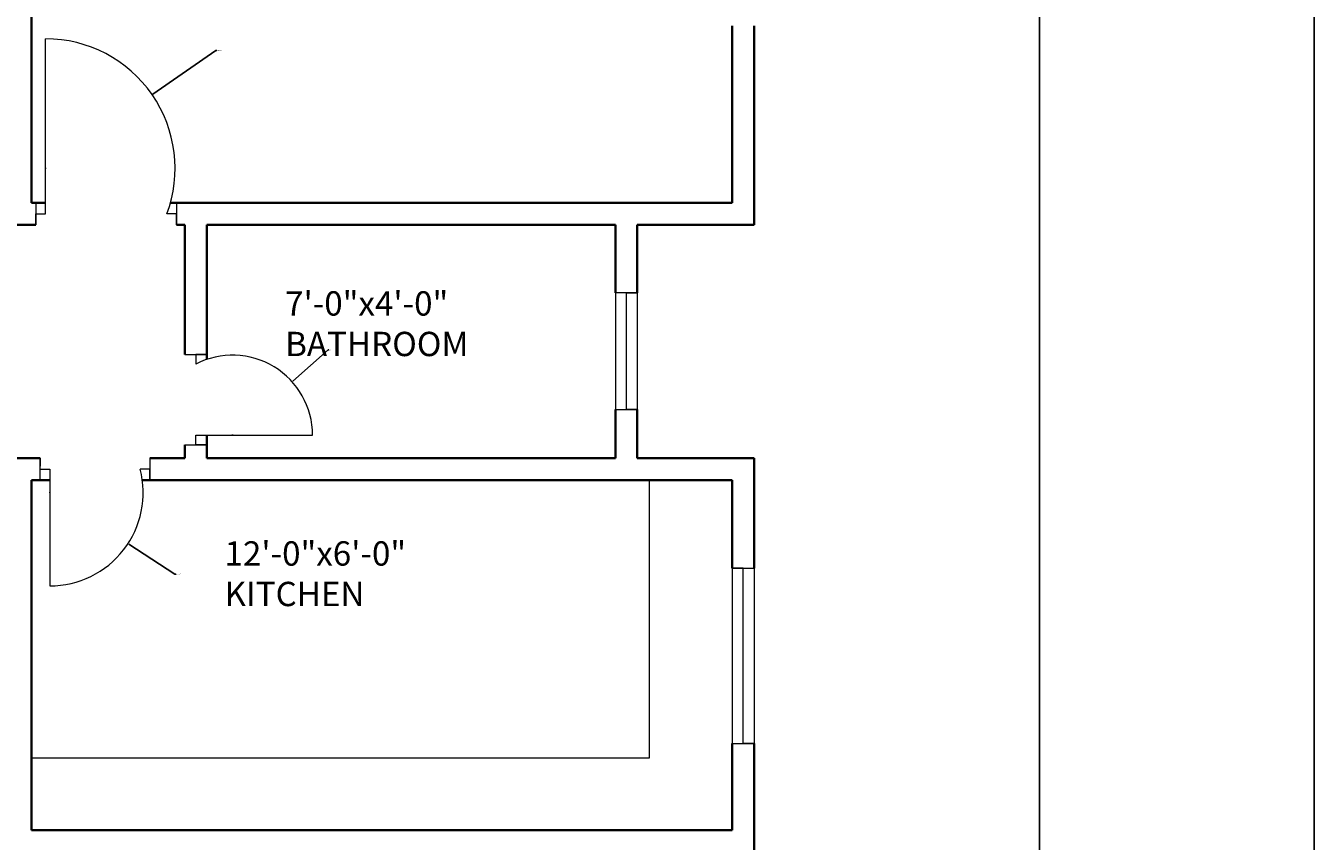
# Model space of a CAD drawing. Units: inches. Extents: x 2163 to 2982, y 1024 to 2288.
# Tile 21 of 22: x 2718 to 2982, y 1885 to 2053. Entities that reach past the tile are written whole.
import ezdxf

# ---------------------------------------------------------------- set-up
doc = ezdxf.new("R2010")
doc.units = ezdxf.units.IN
for name, color, linetype, lineweight in [('A-ANNO-DIMS', 2, 'Continuous', 18), ('A-ANNO-TTLB', 7, 'Continuous', 25), ('A-AREA-IDEN', 7, 'Continuous', 18), ('A-DOOR', 11, 'Continuous', 18), ('A-FLOR-FIXT', 9, 'Continuous', 18), ('A-GLAZ', 161, 'Continuous', 18), ('A-WALL', 7, 'Continuous', 35)]:
    doc.layers.add(name, color=color, linetype=linetype, lineweight=lineweight)
doc.styles.get("Standard").update_dxf_attribs({"font": 'arial.ttf'})
doc.dimstyles.get("Standard").update_dxf_attribs({"dimtxt": 0.18, "dimasz": 0.18, "dimexe": 0.18, "dimexo": 0.0625, "dimgap": 0.09, "dimtad": 0, "dimtih": 1, "dimtoh": 1, "dimdec": 4, "dimzin": 0, "dimdsep": 46, "dimtxsty": 'Standard', "dimcen": 0.09, "dimadec": 0, "dimazin": 0, "dimtfac": 1, "dimtdec": 4, "dimtofl": 0, "dimtmove": 0, "dimatfit": 3, "dimfxl": 1, "dimtolj": 1, "dimtzin": 0, "dimarcsym": 0})

# ---------------------------------------------------------------- blocks, each defined once
blk = doc.blocks.new('WIN-36')
for p, q in [((2.25, 36), (0, 36)), ((0, 36), (4.5, 36)), ((0, 36), (0, 0)), ((2.25, 0), (2.25, 36)), ((4.5, 36), (4.5, 0)), ((0, 0), (4.5, 0)), ((4.5, 0), (2.25, 0))]:
    blk.add_line(p, q)
blk = doc.blocks.new('*D29')
at = {"layer": 'A-ANNO-DIMS', "color": 0, "lineweight": -2, "transparency": 16777216}
for p, q in [((2285.34, 1738.83), (2285.34, 2288.1)), ((2867.34, 2229.33), (2867.34, 2288.1)), ((2285.52, 2287.92), (2576.05, 2287.92)), ((2867.16, 2287.92), (2576.63, 2287.92))]:
    blk.add_line(p, q, dxfattribs=at)
at = {"layer": 'A-ANNO-DIMS', "color": 0, "transparency": 16777216}
for points in [[(2285.52, 2287.95), (2285.52, 2287.89), (2285.34, 2287.92)], [(2867.16, 2287.95), (2867.16, 2287.89), (2867.34, 2287.92)]]:
    blk.add_solid(points, dxfattribs=at)
at = {"layer": 'Defpoints', "color": 0, "transparency": 16777216}
for p in [(2867.34, 2287.92), (2867.34, 2229.27), (2285.34, 1738.77)]:
    blk.add_point(p, dxfattribs=at)
at = {"layer": 'A-ANNO-DIMS', "color": 0, "transparency": 16777216, "insert": (2576.34, 2287.92), "char_height": 0.18, "attachment_point": 5}
blk.add_mtext('\\A1;582', dxfattribs=at)
blk = doc.blocks.new('*D31')
at = {"layer": 'A-ANNO-DIMS', "color": 0, "lineweight": -2, "transparency": 16777216}
for p, q in [((2867.4, 2229.27), (2926.17, 2229.27)), ((2925.99, 2229.09), (2925.99, 1957.95)), ((2925.99, 1686.45), (2925.99, 1957.59)), ((2862.9, 1686.27), (2926.17, 1686.27))]:
    blk.add_line(p, q, dxfattribs=at)
at = {"layer": 'A-ANNO-DIMS', "color": 0, "transparency": 16777216}
for points in [[(2925.96, 2229.09), (2926.02, 2229.09), (2925.99, 2229.27)], [(2925.96, 1686.45), (2926.02, 1686.45), (2925.99, 1686.27)]]:
    blk.add_solid(points, dxfattribs=at)
at = {"layer": 'Defpoints', "color": 0, "transparency": 16777216}
for p in [(2867.34, 2229.27), (2925.99, 2229.27), (2862.84, 1686.27)]:
    blk.add_point(p, dxfattribs=at)
at = {"layer": 'A-ANNO-DIMS', "color": 0, "transparency": 16777216, "insert": (2925.99, 1957.77), "char_height": 0.18, "attachment_point": 5}
blk.add_mtext('\\A1;543', dxfattribs=at)
blk = doc.blocks.new('*D32')
at = {"layer": 'A-ANNO-DIMS', "color": 0, "lineweight": -2, "transparency": 16777216}
for p, q in [((2867.4, 2229.27), (2926.17, 2229.27)), ((2925.99, 2229.09), (2925.99, 1686.35)), ((2925.99, 1143.25), (2925.99, 1685.99)), ((2867.4, 1143.07), (2926.17, 1143.07))]:
    blk.add_line(p, q, dxfattribs=at)
at = {"layer": 'A-ANNO-DIMS', "color": 0, "transparency": 16777216}
for points in [[(2925.96, 2229.09), (2926.02, 2229.09), (2925.99, 2229.27)], [(2925.96, 1143.25), (2926.02, 1143.25), (2925.99, 1143.07)]]:
    blk.add_solid(points, dxfattribs=at)
at = {"layer": 'Defpoints', "color": 0, "transparency": 16777216}
for p in [(2867.34, 2229.27), (2925.99, 2229.27), (2867.34, 1143.07)]:
    blk.add_point(p, dxfattribs=at)
at = {"layer": 'A-ANNO-DIMS', "color": 0, "transparency": 16777216, "insert": (2925.99, 1686.17), "char_height": 0.18, "attachment_point": 5}
blk.add_mtext('\\A1;1086.2', dxfattribs=at)
blk = doc.blocks.new('*D52')
at = {"layer": 'A-ANNO-DIMS', "color": 0, "lineweight": -2, "transparency": 16777216}
for p, q in [((2756.74, 2047.63), (2743.76, 2038.65)), ((2756.92, 2047.63), (2756.74, 2047.63)), ((2721.63, 2023.4), (2721.81, 2023.4)), ((2721.72, 2023.31), (2721.72, 2023.49))]:
    blk.add_line(p, q, dxfattribs=at)
at = {"layer": 'A-ANNO-DIMS', "color": 0, "transparency": 16777216}
blk.add_solid([(2743.74, 2038.67), (2743.78, 2038.62), (2743.61, 2038.55)], dxfattribs=at)
at = {"layer": 'Defpoints', "color": 0, "transparency": 16777216}
for p in [(2743.61, 2038.55), (2721.72, 2023.4)]:
    blk.add_point(p, dxfattribs=at)
at = {"layer": 'A-ANNO-DIMS', "color": 0, "transparency": 16777216, "insert": (2757.47, 2047.63), "char_height": 0.18, "attachment_point": 5}
blk.add_mtext('\\A1;R26.616', dxfattribs=at)
blk = doc.blocks.new('*D70')
at = {"layer": 'A-ANNO-DIMS', "color": 0, "lineweight": -2, "transparency": 16777216}
for p, q in [((2779.77, 1986.04), (2772.55, 1979.6)), ((2779.95, 1986.04), (2779.77, 1986.04)), ((2760.08, 1968.55), (2760.26, 1968.55)), ((2760.17, 1968.46), (2760.17, 1968.64))]:
    blk.add_line(p, q, dxfattribs=at)
at = {"layer": 'A-ANNO-DIMS', "color": 0, "transparency": 16777216}
blk.add_solid([(2772.53, 1979.62), (2772.57, 1979.58), (2772.42, 1979.48)], dxfattribs=at)
at = {"layer": 'Defpoints', "color": 0, "transparency": 16777216}
for p in [(2772.42, 1979.48), (2760.17, 1968.55)]:
    blk.add_point(p, dxfattribs=at)
at = {"layer": 'A-ANNO-DIMS', "color": 0, "transparency": 16777216, "insert": (2780.5, 1986.04), "char_height": 0.18, "attachment_point": 5}
blk.add_mtext('\\A1;R16.423', dxfattribs=at)
blk = doc.blocks.new('*D72')
at = {"layer": 'A-ANNO-DIMS', "color": 0, "lineweight": -2, "transparency": 16777216}
for p, q in [((2722.5, 1956.72), (2722.68, 1956.72)), ((2722.59, 1956.63), (2722.59, 1956.81)), ((2748.31, 1939.92), (2738.81, 1946.12)), ((2748.49, 1939.92), (2748.31, 1939.92))]:
    blk.add_line(p, q, dxfattribs=at)
at = {"layer": 'A-ANNO-DIMS', "color": 0, "transparency": 16777216}
blk.add_solid([(2738.83, 1946.15), (2738.8, 1946.1), (2738.66, 1946.22)], dxfattribs=at)
at = {"layer": 'Defpoints', "color": 0, "transparency": 16777216}
for p in [(2722.59, 1956.72), (2738.66, 1946.22)]:
    blk.add_point(p, dxfattribs=at)
at = {"layer": 'A-ANNO-DIMS', "color": 0, "transparency": 16777216, "insert": (2749.04, 1939.92), "char_height": 0.18, "attachment_point": 5}
blk.add_mtext('\\A1;R19.197', dxfattribs=at)

msp = doc.modelspace()

# ---------------------------------------------------------------- linework, layer by layer
at = {"layer": 'A-ANNO-TTLB'}
msp.add_lwpolyline([(2162.6841, 2274.6054), (2982.469, 2274.6054), (2982.469, 1045.9691), (2162.6841, 1045.9691)], close=True, dxfattribs=at)
at = {"layer": 'A-DOOR'}
for p, q in [((2721.7236, 2014.0188), (2721.7236, 2050.0188)), ((2719.7237, 2016.2688), (2719.7237, 2011.7688)), ((2748.6306, 2016.2688), (2748.6306, 2011.7688)), ((2719.7237, 2011.7688), (2719.7237, 2014.0188)), ((2719.7237, 2014.0188), (2721.7236, 2014.0188)), ((2748.6306, 2014.0188), (2746.6306, 2014.0188)), ((2748.6306, 2011.7688), (2748.6306, 2014.0188)), ((2750.3389, 1985.1163), (2754.8389, 1985.1163)), ((2754.8389, 1985.1163), (2752.5889, 1985.1163)), ((2752.5889, 1985.1163), (2752.5889, 1983.1163)), ((2752.5889, 1966.5459), (2752.5889, 1968.5459)), ((2752.5889, 1968.5459), (2776.5889, 1968.5459)), ((2750.3389, 1966.5459), (2754.8389, 1966.5459)), ((2754.8389, 1966.5459), (2752.5889, 1966.5459)), ((2720.5891, 1959.2688), (2720.5891, 1963.7688)), ((2720.5891, 1963.7688), (2720.5891, 1962.1629)), ((2743.1754, 1963.7688), (2743.1754, 1959.2688)), ((2720.5891, 1961.5188), (2722.5891, 1961.5188)), ((2722.5891, 1961.5188), (2722.5891, 1937.5188)), ((2743.1754, 1961.5188), (2741.1754, 1961.5188)), ((2743.1754, 1959.2688), (2743.1754, 1961.5188))]:
    msp.add_line(p, q, dxfattribs=at)
for centre, radius, start, end in [((2721.7236, 2023.4028), 26.6161, 339.35562, 90), ((2760.1661, 1968.5459), 16.4228, 0, 117.476424), ((2722.5891, 1956.7157), 19.1969, 270, 14.489541)]:
    msp.add_arc(centre, radius, start, end, dxfattribs=at)
at = {"layer": 'A-FLOR-FIXT'}
for p, q in [((2845.79, 1959.2688), (2845.79, 1902.0881)), ((2845.79, 1902.0881), (2718.8389, 1902.0881))]:
    msp.add_line(p, q, dxfattribs=at)
at = {"layer": 'A-GLAZ'}
for p, q in [((2843.3389, 1997.762), (2838.8389, 1997.762)), ((2838.8389, 1997.762), (2838.8389, 1973.762)), ((2841.0889, 1973.762), (2841.0889, 1997.762)), ((2841.0889, 1997.762), (2843.3389, 1997.762)), ((2843.3389, 1997.762), (2843.3389, 1973.762)), ((2838.8389, 1973.762), (2843.3389, 1973.762)), ((2843.3389, 1973.762), (2841.0889, 1973.762))]:
    msp.add_line(p, q, dxfattribs=at)
at = {"layer": 'A-WALL'}
for p, q in [((2718.8389, 2172.2688), (2718.8389, 2016.2688)), ((2862.8389, 2052.7024), (2862.8389, 2016.2688)), ((2867.3389, 2052.7024), (2867.3389, 2011.7688)), ((2718.8389, 2016.2688), (2721.7236, 2016.2688)), ((2747.3658, 2016.2688), (2862.8389, 2016.2688)), ((2620.9736, 2011.7688), (2718.8389, 2011.7688)), ((2718.8389, 2011.7688), (2719.7237, 2011.7688)), ((2748.6306, 2011.7688), (2750.3389, 2011.7688)), ((2750.3389, 2011.7688), (2750.3389, 1985.1163)), ((2834.3389, 2011.7688), (2754.8389, 2011.7688)), ((2838.8389, 2011.7688), (2754.8389, 2011.7688)), ((2754.8389, 2011.7688), (2838.8389, 2011.7688)), ((2754.8389, 1984.0807), (2754.8389, 2011.7688)), ((2838.8389, 2011.7688), (2838.8389, 1997.762)), ((2862.8389, 2011.7688), (2843.3389, 2011.7688)), ((2843.3389, 2011.7688), (2843.3389, 1997.762)), ((2843.3389, 2011.7688), (2867.3389, 2011.7688)), ((2838.8389, 1973.762), (2838.8389, 1963.7688)), ((2843.3389, 1973.762), (2843.3389, 1963.7688)), ((2754.8389, 1963.7688), (2754.8389, 1968.5459)), ((2750.3389, 1966.5459), (2750.3389, 1963.7688)), ((2714.3389, 1963.7688), (2720.5891, 1963.7688)), ((2743.1754, 1963.7688), (2750.3389, 1963.7688)), ((2754.8389, 1963.7688), (2838.8389, 1963.7688)), ((2838.8389, 1963.7688), (2834.3389, 1963.7688)), ((2843.3389, 1963.7688), (2867.3389, 1963.7688)), ((2867.3389, 1963.7688), (2867.3389, 1941.1374)), ((2718.8389, 1959.2688), (2722.5891, 1959.2688)), ((2718.8389, 1959.2688), (2718.8389, 1887.2688)), ((2741.6155, 1959.2688), (2862.8389, 1959.2688)), ((2862.8389, 1959.2688), (2862.8389, 1941.1374)), ((2862.8389, 1905.1374), (2862.8389, 1887.2688)), ((2867.3389, 1905.1374), (2867.3389, 1882.7688)), ((2718.8389, 1887.2688), (2862.8389, 1887.2688))]:
    msp.add_line(p, q, dxfattribs=at)

# ---------------------------------------------------------------- block references
at = {"layer": 'A-GLAZ'}
msp.add_blockref('WIN-36', (2862.839, 1905.137), dxfattribs=at)

# ---------------------------------------------------------------- texts
at = {"layer": 'A-AREA-IDEN', "char_height": 5, "attachment_point": 1}
for s, width, insert in [('7\'-0"x4\'-0"\\PBATHROOM', 46.485545, (2770.9551, 1998.1065)), ('12\'-0"x6\'-0"\\PKITCHEN', 101.55276, (2758.5046, 1946.6966))]:
    msp.add_mtext_dynamic_manual_height_columns(s, width=width, gutter_width=12.5, heights=[0], dxfattribs=dict(at, insert=insert))

# ---------------------------------------------------------------- dimensions: what is measured, and where the dimension line sits
at = {"layer": 'A-ANNO-DIMS'}
dim = msp.add_linear_dim(base=(2867.3389, 2287.9188), p1=(2285.3389, 1738.7688), p2=(2867.3389, 2229.2688), dimstyle='Standard', override={"dimdec": 0, "dimlfac": 1, "dimrnd": 0, "dimzin": 0, "dimdsep": 46, "dimlunit": 2}, dxfattribs=at)
dim.commit()
dim.dimension.update_dxf_attribs({"geometry": '*D29', "text_midpoint": (2576.3389, 2287.9188)})
for p1, override, picture, middle in [((2862.8389, 1686.2688), {"dimdec": 0, "dimlfac": 1, "dimrnd": 0, "dimzin": 0, "dimdsep": 46, "dimlunit": 2}, '*D31', (2925.9889, 1957.7688)), ((2867.3389, 1143.0732), {"dimdec": 1, "dimlfac": 1, "dimrnd": 0, "dimzin": 0, "dimdsep": 46, "dimlunit": 2}, '*D32', (2925.9889, 1686.171))]:
    dim = msp.add_linear_dim(base=(2925.9889, 2229.2688), p1=p1, p2=(2867.3389, 2229.2688), angle=90, dimstyle='Standard', override=override, dxfattribs=at)
    dim.commit()
    dim.dimension.update_dxf_attribs({"geometry": picture, "text_midpoint": middle})
for center, mpoint, picture, middle in [((2721.7236, 2023.4028), (2743.612, 2038.546), '*D52', (2757.4747, 2047.6319)), ((2760.1661, 1968.5459), (2772.4188, 1979.4813), '*D70', (2780.5001, 1986.0424)), ((2722.5891, 1956.7157), (2738.6628, 1946.2202), '*D72', (2749.0368, 1939.9228))]:
    dim = msp.add_radius_dim(center=center, mpoint=mpoint, dimstyle='Standard', override={"dimdec": 3, "dimlfac": 1, "dimrnd": 0, "dimzin": 0, "dimdsep": 46, "dimlunit": 2}, dxfattribs=at)
    dim.commit()
    dim.dimension.update_dxf_attribs({"geometry": picture, "text_midpoint": middle, "dimtype": 164})

doc.saveas('drawing.dxf')
